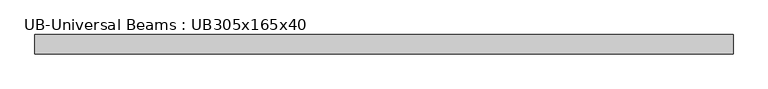
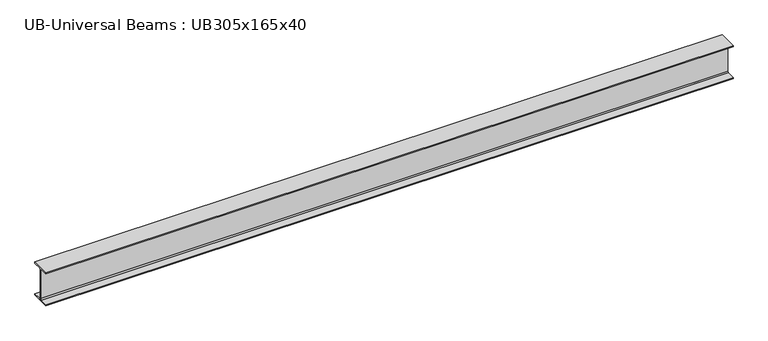
"""IFC4 building model written with IfcOpenShell, lengths in millimetres: beam geometry, UB-Universal Beams : UB305x165x40."""

from ifc_helpers import new_model, si_unit, point, frame, frame_2d, origin, place, context, project, spatial, polyline, circle_curve, trimmed, segment, composite_curve, outline, extrude, source, transform, mapped, element, save


def ub_universal_beams_ub305x165x40_694d595e(model_context):
    return source(origin(), model_context, "Body", "SweptSolid", [
        extrude(outline(composite_curve([segment(polyline([(82.5, -141.5), (82.5, -151.7), (-82.5, -151.7), (-82.5, -141.5), (-11.9, -141.5)]), True, "CONTINUOUS"), segment(trimmed(circle_curve(frame_2d((-11.9, -132.6)), 8.9), [point((-11.9, -141.5))], [point((-3.0, -132.6))], True, "CARTESIAN"), True, "CONTINUOUS"), segment(polyline([(-3.0, -132.6), (-3.0, 132.6)]), True, "CONTINUOUS"), segment(trimmed(circle_curve(frame_2d((-11.9, 132.6)), 8.9), [point((-3.0, 132.6))], [point((-11.9, 141.5))], True, "CARTESIAN"), True, "CONTINUOUS"), segment(polyline([(-11.9, 141.5), (-82.5, 141.5), (-82.5, 151.7), (82.5, 151.7), (82.5, 141.5), (11.9, 141.5)]), True, "CONTINUOUS"), segment(trimmed(circle_curve(frame_2d((11.9, 132.6)), 8.9), [point((11.9, 141.5))], [point((3.0, 132.6))], True, "CARTESIAN"), True, "CONTINUOUS"), segment(polyline([(3.0, 132.6), (3.0, -132.6)]), True, "CONTINUOUS"), segment(trimmed(circle_curve(frame_2d((11.9, -132.6)), 8.9), [point((3.0, -132.6))], [point((11.9, -141.5))], True, "CARTESIAN"), True, "CONTINUOUS"), segment(polyline([(11.9, -141.5), (82.5, -141.5)]), True, "CONTINUOUS")], self_intersect=False)), frame((-2978.15, 0.0, 0.0), z_axis=(1.0, 0.0, 0.0), x_axis=(0.0, 1.0, 0.0)), (0.0, 0.0, 1.0), 5988.1),
    ])


if __name__ == "__main__":
    model = new_model("IFC4")
    model_context = context("Model", 3, world=origin())
    ifc_project = project(units=[si_unit("LENGTHUNIT", "METRE", prefix="MILLI")], contexts=[model_context])
    site = spatial("IfcSite", under=ifc_project)
    building = spatial("IfcBuilding", under=site)
    placement = place(None, origin())
    ub_universal_beams_ub305x165x40_shape = ub_universal_beams_ub305x165x40_694d595e(model_context)
    element("IfcBeam", 1, ObjectType="UB-Universal Beams : UB305x165x40", at=placement, inside=building, context=model_context, shape_type="MappedRepresentation", body=[
        mapped(ub_universal_beams_ub305x165x40_shape, transform((0.0, 0.0, 0.0), x_axis=(1.0, 0.0, 0.0), y_axis=(0.0, 1.0, 0.0), z_axis=(0.0, 0.0, 1.0))),
    ])
    save(model, "model.ifc")

# Revit data of these elements
# Type "UB-Universal Beams : UB305x165x40"
#   Section Name Key = "UB305X165X40"
#   Width = 16.5 cm
#   Web Thickness = 0.6 cm
#   Web Fillet = 0.89 cm
#   Warping Constant = 164000.0 cm⁶
#   Torsional Moment of Inertia = 14.70 cm⁴
#   Section Area = 51.3 cm²
#   Plastic Modulus weak axis = 142.0 cm³
#   Plastic Modulus strong axis = 623.0 cm³
#   Nominal Weight = 40.2999 kgf/m
#   Moment of Inertia weak axis = 764.00 cm⁴
#   Moment of Inertia strong axis = 8503.00 cm⁴
#   Height = 30.34 cm
#   Flange Thickness = 1.02 cm
#   Elastic Modulus weak axis = 92.6 cm³
#   Elastic Modulus strong axis = 560.0 cm³
#   Centroid Vertical = 15.17 cm
#   Centroid Horizontal = 8.25 cm
#   Bolt Spacing = 9.0 cm
#   Length [instance default] = 1500 mm
#   Structural Material [instance default] = Metal - Steel 43-275
#   Type Comments = ""
#   Assembly Code = ""
# Element 1 (IfcBeam, "UB-Universal Beams : UB305x165x40")
#   Materials on its faces: "Metal - Steel 43-275"
# Materials
#   "Metal - Steel 43-275": class "Metal", colour RGB 247 247 247, transparency 0, Cost = 0
